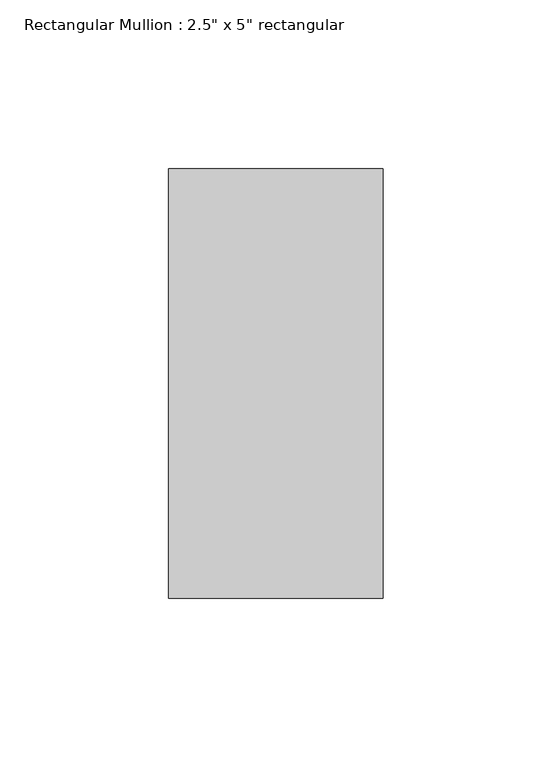
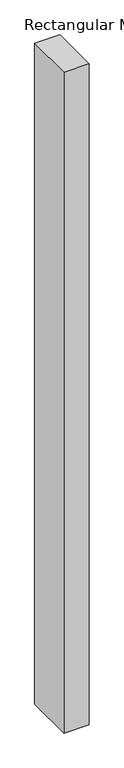
"""IFC4 building model written with IfcOpenShell, lengths in millimetres: member geometry."""

from ifc_helpers import new_model, si_unit, frame, origin, place, context, project, spatial, polyline, outline, extrude, source, transform, mapped, element, save


def member_e7b07674(model_context):
    return source(origin(), model_context, "Body", "SweptSolid", [
        extrude(outline(polyline([(31.75, 63.5), (31.75, -63.5), (-31.75, -63.5), (-31.75, 63.5), (31.75, 63.5)])), frame((0.0, 0.0, -1757.2747989), z_axis=(0.0, 0.0, 1.0), x_axis=(1.0, 0.0, 0.0)), (0.0, 0.0, 1.0), 1757.2747989),
    ])


if __name__ == "__main__":
    model = new_model("IFC4")
    model_context = context("Model", 3, world=origin())
    ifc_project = project(units=[si_unit("LENGTHUNIT", "METRE", prefix="MILLI")], contexts=[model_context])
    site = spatial("IfcSite", under=ifc_project)
    building = spatial("IfcBuilding", under=site)
    placement = place(None, origin())
    member_shape = member_e7b07674(model_context)
    element("IfcMember", 1, ObjectType="Rectangular Mullion : 2.5\" x 5\" rectangular", at=placement, inside=building, context=model_context, shape_type="MappedRepresentation", body=[
        mapped(member_shape, transform((0.0, 0.0, 0.0), x_axis=(1.0, 0.0, 0.0), y_axis=(0.0, 1.0, 0.0), z_axis=(0.0, 0.0, 1.0))),
    ])
    save(model, "model.ifc")

# Revit data of these elements
# Type "Rectangular Mullion : 2.5\" x 5\" rectangular"
#   built-in parameter 1007304 = 0.416667 (stored number, unit not read)
#   built-in parameter 1007301 = 0.104167 (stored number, unit not read)
#   built-in parameter 1007300 = 0.104167 (stored number, unit not read)
# Element 1 (IfcMember, "Rectangular Mullion : 2.5\" x 5\" rectangular")
#   Materials on its faces: "Aluminum"
# Materials
#   "Aluminum": class "Metal", colour RGB 247 247 247, transparency 0, Description = "Aluminum 6061", Cost = 0
